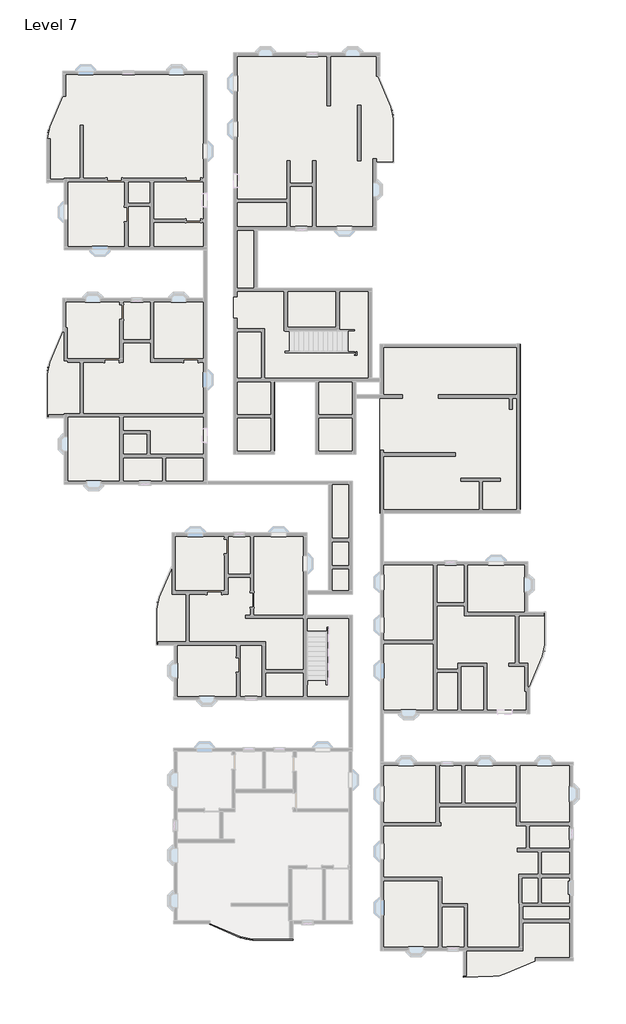
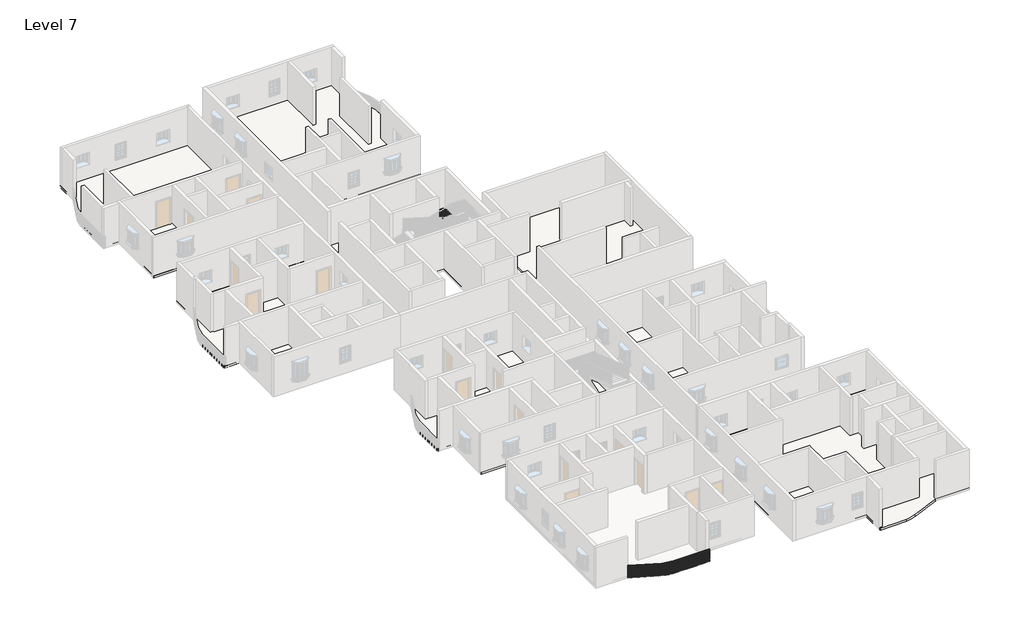
# One storey, part 5 of 14: 24 roofs, 1 railing.
"""IFC4 building model written with IfcOpenShell, lengths in millimetres."""

from ifc_helpers import new_model, si_unit, point, frame, frame_2d, origin, place, context, project, spatial, polyline, circle_curve, trimmed, segment, composite_curve, outline, extrude, element, save
from ifc_brep_helpers import plane_surface, cylinder_surface, revolved_surface, advanced_brep

model = new_model("IFC4")

# Units and contexts
model_context = context("Model", 3, world=origin())
ifc_project = project(units=[si_unit("LENGTHUNIT", "METRE", prefix="MILLI")], contexts=[model_context])

# Site, building, storey
site = spatial("IfcSite", under=ifc_project)
building = spatial("IfcBuilding", under=site)
storey = spatial("IfcBuildingStorey", under=building, Name="Level 7", Elevation=18288.0)

# Railing
placement = place(None, origin())
element("IfcRailing", 1, ObjectType="Handrail - Rectangular", at=placement, inside=storey, context=model_context, shape_type="SolidModel", body=[
    advanced_brep(
    [(-10014.8722294, -25076.9923935, 19202.4), (-10014.8722294, -25076.9923935, 19151.6), (-10034.8694485, -25123.6909077, 19151.6), (-10034.8694485, -25123.6909077, 19202.4), (-8065.5370278, -25911.7359335, 19202.4), (-8065.5370278, -25911.7359335, 19151.6), (-8085.5342469, -25958.4344477, 19151.6), (-8085.5342469, -25958.4344477, 19202.4), (-7315.6413127, -26065.5416506, 19151.6), (-7315.6413127, -26065.5416506, 19202.4), (-7315.6413127, -26116.3416506, 19151.6), (-7315.6413127, -26116.3416506, 19202.4), (-4746.0891351, -26065.5416506, 19202.4), (-4746.0891351, -26116.3416506, 19202.4), (-4746.0891351, -26116.3416506, 19151.6), (-4746.0891351, -26065.5416506, 19151.6)],
    [
        (0, 1),
        (1, 2),
        (2, 3),
        (3, 0),
        (0, 4),
        (4, 5),
        (5, 1),
        (5, 6),
        (6, 2),
        (6, 7),
        (7, 3),
        (7, 4),
        (8, 5, circle_curve(frame((-7315.6413127, -24160.5416506, 19151.6), z_axis=(0.0, 0.0, -1.0), x_axis=(-0.3936460446736572, -0.9192620907623599, 0.0)), 1905.0)),
        (4, 9, circle_curve(frame((-7315.6413127, -24160.5416506, 19202.4), z_axis=(0.0, 0.0, 1.0), x_axis=(-0.3936460446736572, -0.9192620907623599, 0.0)), 1905.0)),
        (9, 8),
        (10, 6, circle_curve(frame((-7315.6413127, -24160.5416506, 19151.6), z_axis=(0.0, 0.0, -1.0), x_axis=(-0.3936460446736572, -0.9192620907623599, 0.0)), 1955.8)),
        (8, 10),
        (11, 7, circle_curve(frame((-7315.6413127, -24160.5416506, 19202.4), z_axis=(0.0, 0.0, -1.0), x_axis=(-0.3936460446736572, -0.9192620907623599, 0.0)), 1955.8)),
        (10, 11),
        (11, 9),
        (12, 13),
        (13, 14),
        (14, 15),
        (15, 12),
        (9, 12),
        (15, 8),
        (14, 10),
        (13, 11),
    ],
    [
        plane_surface(frame((-10024.8708389, -25100.3416506, 19202.4), z_axis=(-0.9192620907623597, 0.39364604467365766, 0.0), x_axis=(0.39364604467365766, 0.9192620907623597, 0.0))),
        plane_surface(frame((-10014.8722294, -25076.9923935, 19202.4), z_axis=(0.3936460446736573, 0.9192620907623599, 0.0), x_axis=(0.9192620907623599, -0.3936460446736573, 0.0))),
        plane_surface(frame((-10014.8722294, -25076.9923935, 19151.6), z_axis=(0.0, 0.0, -1.0000000000000002), x_axis=(0.9192620907623599, -0.3936460446736573, 0.0))),
        plane_surface(frame((-10034.8694485, -25123.6909077, 19151.6), z_axis=(-0.39364604467365766, -0.9192620907623597, 0.0), x_axis=(0.9192620907623597, -0.39364604467365766, 0.0))),
        plane_surface(frame((-10034.8694485, -25123.6909077, 19202.4), z_axis=(0.0, 0.0, 1.0), x_axis=(0.9192620907623597, -0.39364604467365766, 0.0))),
        revolved_surface(polyline([(-8065.537027803317, -25911.735933502296, 19202.4), (-8065.537027803317, -25911.735933502296, 19151.6)]), (-7315.6413127, -24160.5416506, 19202.4), (0.0, 0.0, 1.0)),
        plane_surface(frame((-7315.6413127, -24160.5416506, 19151.6), z_axis=(0.0, 0.0, -1.0), x_axis=(-0.3936460446736572, -0.9192620907623599, 0.0))),
        cylinder_surface(frame((-7315.6413127, -24160.5416506, 19202.4), z_axis=(0.0, 0.0, 1.0), x_axis=(-0.3936460446736572, -0.9192620907623599, 0.0)), 1955.8),
        plane_surface(frame((-7315.6413127, -24160.5416506, 19202.4), z_axis=(0.0, 0.0, 1.0), x_axis=(-0.3936460446736572, -0.9192620907623599, 0.0))),
        plane_surface(frame((-4746.0891351, -26090.9416506, 19202.4), z_axis=(1.0, 0.0, 0.0), x_axis=(0.0, 1.0, 0.0))),
        plane_surface(frame((-7315.6413127, -26065.5416506, 19202.4), z_axis=(0.0, 1.0, 0.0), x_axis=(1.0, 0.0, 0.0))),
        plane_surface(frame((-7315.6413127, -26065.5416506, 19151.6), z_axis=(0.0, 0.0, -1.0), x_axis=(1.0, 0.0, 0.0))),
        plane_surface(frame((-7315.6413127, -26116.3416506, 19151.6), z_axis=(0.0, -1.0, 0.0), x_axis=(1.0, 0.0, 0.0))),
        plane_surface(frame((-7315.6413127, -26116.3416506, 19202.4), z_axis=(0.0, 0.0, 1.0), x_axis=(1.0, 0.0, 0.0))),
    ],
    [
        (0, [[1, 2, 3, 4]]),
        (1, [[-1, 5, 6, 7]]),
        (2, [[-2, -7, 8, 9]]),
        (3, [[-3, -9, 10, 11]]),
        (4, [[-4, -11, 12, -5]]),
        (5, [[13, -6, 14, 15]]),
        (6, [[16, -8, -13, 17]]),
        (7, [[18, -10, -16, 19]]),
        (8, [[-14, -12, -18, 20]]),
        (9, [[21, 22, 23, 24]]),
        (10, [[-15, 25, -24, 26]]),
        (11, [[-17, -26, -23, 27]]),
        (12, [[-19, -27, -22, 28]]),
        (13, [[-20, -28, -21, -25]]),
    ],
),
    extrude(outline(polyline([(-4785.1663127, -26100.4666506), (-4785.1663127, -26081.4166506), (-4766.1163127, -26081.4166506), (-4766.1163127, -26100.4666506), (-4785.1663127, -26100.4666506)])), frame((0.0, 0.0, 18288.0), z_axis=(0.0, 0.0, 1.0), x_axis=(1.0, 0.0, 0.0)), (0.0, 0.0, 1.0), 863.6),
    extrude(outline(polyline([(-4886.7663127, -26100.4666506), (-4886.7663127, -26081.4166506), (-4867.7163127, -26081.4166506), (-4867.7163127, -26100.4666506), (-4886.7663127, -26100.4666506)])), frame((0.0, 0.0, 18288.0), z_axis=(0.0, 0.0, 1.0), x_axis=(1.0, 0.0, 0.0)), (0.0, 0.0, 1.0), 863.6),
    extrude(outline(polyline([(-4988.3663127, -26100.4666506), (-4988.3663127, -26081.4166506), (-4969.3163127, -26081.4166506), (-4969.3163127, -26100.4666506), (-4988.3663127, -26100.4666506)])), frame((0.0, 0.0, 18288.0), z_axis=(0.0, 0.0, 1.0), x_axis=(1.0, 0.0, 0.0)), (0.0, 0.0, 1.0), 863.6),
    extrude(outline(polyline([(-5089.9663127, -26100.4666506), (-5089.9663127, -26081.4166506), (-5070.9163127, -26081.4166506), (-5070.9163127, -26100.4666506), (-5089.9663127, -26100.4666506)])), frame((0.0, 0.0, 18288.0), z_axis=(0.0, 0.0, 1.0), x_axis=(1.0, 0.0, 0.0)), (0.0, 0.0, 1.0), 863.6),
    extrude(outline(polyline([(-5191.5663127, -26100.4666506), (-5191.5663127, -26081.4166506), (-5172.5163127, -26081.4166506), (-5172.5163127, -26100.4666506), (-5191.5663127, -26100.4666506)])), frame((0.0, 0.0, 18288.0), z_axis=(0.0, 0.0, 1.0), x_axis=(1.0, 0.0, 0.0)), (0.0, 0.0, 1.0), 863.6),
    extrude(outline(polyline([(-5293.1663127, -26100.4666506), (-5293.1663127, -26081.4166506), (-5274.1163127, -26081.4166506), (-5274.1163127, -26100.4666506), (-5293.1663127, -26100.4666506)])), frame((0.0, 0.0, 18288.0), z_axis=(0.0, 0.0, 1.0), x_axis=(1.0, 0.0, 0.0)), (0.0, 0.0, 1.0), 863.6),
    extrude(outline(polyline([(-5394.7663127, -26100.4666506), (-5394.7663127, -26081.4166506), (-5375.7163127, -26081.4166506), (-5375.7163127, -26100.4666506), (-5394.7663127, -26100.4666506)])), frame((0.0, 0.0, 18288.0), z_axis=(0.0, 0.0, 1.0), x_axis=(1.0, 0.0, 0.0)), (0.0, 0.0, 1.0), 863.6),
    extrude(outline(polyline([(-5496.3663127, -26100.4666506), (-5496.3663127, -26081.4166506), (-5477.3163127, -26081.4166506), (-5477.3163127, -26100.4666506), (-5496.3663127, -26100.4666506)])), frame((0.0, 0.0, 18288.0), z_axis=(0.0, 0.0, 1.0), x_axis=(1.0, 0.0, 0.0)), (0.0, 0.0, 1.0), 863.6),
    extrude(outline(polyline([(-5597.9663127, -26100.4666506), (-5597.9663127, -26081.4166506), (-5578.9163127, -26081.4166506), (-5578.9163127, -26100.4666506), (-5597.9663127, -26100.4666506)])), frame((0.0, 0.0, 18288.0), z_axis=(0.0, 0.0, 1.0), x_axis=(1.0, 0.0, 0.0)), (0.0, 0.0, 1.0), 863.6),
    extrude(outline(polyline([(-5699.5663127, -26100.4666506), (-5699.5663127, -26081.4166506), (-5680.5163127, -26081.4166506), (-5680.5163127, -26100.4666506), (-5699.5663127, -26100.4666506)])), frame((0.0, 0.0, 18288.0), z_axis=(0.0, 0.0, 1.0), x_axis=(1.0, 0.0, 0.0)), (0.0, 0.0, 1.0), 863.6),
    extrude(outline(polyline([(-5801.1663127, -26100.4666506), (-5801.1663127, -26081.4166506), (-5782.1163127, -26081.4166506), (-5782.1163127, -26100.4666506), (-5801.1663127, -26100.4666506)])), frame((0.0, 0.0, 18288.0), z_axis=(0.0, 0.0, 1.0), x_axis=(1.0, 0.0, 0.0)), (0.0, 0.0, 1.0), 863.6),
    extrude(outline(polyline([(-5902.7663127, -26100.4666506), (-5902.7663127, -26081.4166506), (-5883.7163127, -26081.4166506), (-5883.7163127, -26100.4666506), (-5902.7663127, -26100.4666506)])), frame((0.0, 0.0, 18288.0), z_axis=(0.0, 0.0, 1.0), x_axis=(1.0, 0.0, 0.0)), (0.0, 0.0, 1.0), 863.6),
    extrude(outline(polyline([(-6004.3663127, -26100.4666506), (-6004.3663127, -26081.4166506), (-5985.3163127, -26081.4166506), (-5985.3163127, -26100.4666506), (-6004.3663127, -26100.4666506)])), frame((0.0, 0.0, 18288.0), z_axis=(0.0, 0.0, 1.0), x_axis=(1.0, 0.0, 0.0)), (0.0, 0.0, 1.0), 863.6),
    extrude(outline(polyline([(-6105.9663127, -26100.4666506), (-6105.9663127, -26081.4166506), (-6086.9163127, -26081.4166506), (-6086.9163127, -26100.4666506), (-6105.9663127, -26100.4666506)])), frame((0.0, 0.0, 18288.0), z_axis=(0.0, 0.0, 1.0), x_axis=(1.0, 0.0, 0.0)), (0.0, 0.0, 1.0), 863.6),
    extrude(outline(polyline([(-6207.5663127, -26100.4666506), (-6207.5663127, -26081.4166506), (-6188.5163127, -26081.4166506), (-6188.5163127, -26100.4666506), (-6207.5663127, -26100.4666506)])), frame((0.0, 0.0, 18288.0), z_axis=(0.0, 0.0, 1.0), x_axis=(1.0, 0.0, 0.0)), (0.0, 0.0, 1.0), 863.6),
    extrude(outline(polyline([(-6309.1663127, -26100.4666506), (-6309.1663127, -26081.4166506), (-6290.1163127, -26081.4166506), (-6290.1163127, -26100.4666506), (-6309.1663127, -26100.4666506)])), frame((0.0, 0.0, 18288.0), z_axis=(0.0, 0.0, 1.0), x_axis=(1.0, 0.0, 0.0)), (0.0, 0.0, 1.0), 863.6),
    extrude(outline(polyline([(-6410.7663127, -26100.4666506), (-6410.7663127, -26081.4166506), (-6391.7163127, -26081.4166506), (-6391.7163127, -26100.4666506), (-6410.7663127, -26100.4666506)])), frame((0.0, 0.0, 18288.0), z_axis=(0.0, 0.0, 1.0), x_axis=(1.0, 0.0, 0.0)), (0.0, 0.0, 1.0), 863.6),
    extrude(outline(polyline([(-6512.3663127, -26100.4666506), (-6512.3663127, -26081.4166506), (-6493.3163127, -26081.4166506), (-6493.3163127, -26100.4666506), (-6512.3663127, -26100.4666506)])), frame((0.0, 0.0, 18288.0), z_axis=(0.0, 0.0, 1.0), x_axis=(1.0, 0.0, 0.0)), (0.0, 0.0, 1.0), 863.6),
    extrude(outline(polyline([(-6613.9663127, -26100.4666506), (-6613.9663127, -26081.4166506), (-6594.9163127, -26081.4166506), (-6594.9163127, -26100.4666506), (-6613.9663127, -26100.4666506)])), frame((0.0, 0.0, 18288.0), z_axis=(0.0, 0.0, 1.0), x_axis=(1.0, 0.0, 0.0)), (0.0, 0.0, 1.0), 863.6),
    extrude(outline(polyline([(-6715.5663127, -26100.4666506), (-6715.5663127, -26081.4166506), (-6696.5163127, -26081.4166506), (-6696.5163127, -26100.4666506), (-6715.5663127, -26100.4666506)])), frame((0.0, 0.0, 18288.0), z_axis=(0.0, 0.0, 1.0), x_axis=(1.0, 0.0, 0.0)), (0.0, 0.0, 1.0), 863.6),
    extrude(outline(polyline([(-6817.1663127, -26100.4666506), (-6817.1663127, -26081.4166506), (-6798.1163127, -26081.4166506), (-6798.1163127, -26100.4666506), (-6817.1663127, -26100.4666506)])), frame((0.0, 0.0, 18288.0), z_axis=(0.0, 0.0, 1.0), x_axis=(1.0, 0.0, 0.0)), (0.0, 0.0, 1.0), 863.6),
    extrude(outline(polyline([(-6918.7663127, -26100.4666506), (-6918.7663127, -26081.4166506), (-6899.7163127, -26081.4166506), (-6899.7163127, -26100.4666506), (-6918.7663127, -26100.4666506)])), frame((0.0, 0.0, 18288.0), z_axis=(0.0, 0.0, 1.0), x_axis=(1.0, 0.0, 0.0)), (0.0, 0.0, 1.0), 863.6),
    extrude(outline(polyline([(-7020.3663127, -26100.4666506), (-7020.3663127, -26081.4166506), (-7001.3163127, -26081.4166506), (-7001.3163127, -26100.4666506), (-7020.3663127, -26100.4666506)])), frame((0.0, 0.0, 18288.0), z_axis=(0.0, 0.0, 1.0), x_axis=(1.0, 0.0, 0.0)), (0.0, 0.0, 1.0), 863.6),
    extrude(outline(polyline([(-7121.9663127, -26100.4666506), (-7121.9663127, -26081.4166506), (-7102.9163127, -26081.4166506), (-7102.9163127, -26100.4666506), (-7121.9663127, -26100.4666506)])), frame((0.0, 0.0, 18288.0), z_axis=(0.0, 0.0, 1.0), x_axis=(1.0, 0.0, 0.0)), (0.0, 0.0, 1.0), 863.6),
    extrude(outline(polyline([(-7223.5663127, -26100.4666506), (-7223.5663127, -26081.4166506), (-7204.5163127, -26081.4166506), (-7204.5163127, -26100.4666506), (-7223.5663127, -26100.4666506)])), frame((0.0, 0.0, 18288.0), z_axis=(0.0, 0.0, 1.0), x_axis=(1.0, 0.0, 0.0)), (0.0, 0.0, 1.0), 863.6),
    extrude(outline(polyline([(-7395.3185803, -26098.8530973), (-7394.6296262, -26079.8155596), (-7375.5920885, -26080.5045137), (-7376.2810426, -26099.5420514), (-7395.3185803, -26098.8530973)])), frame((0.0, 0.0, 18288.0), z_axis=(0.0, 0.0, 1.0), x_axis=(1.0, 0.0, 0.0)), (0.0, 0.0, 1.0), 863.6),
    extrude(outline(polyline([(-7497.177549, -26091.9774704), (-7495.4880357, -26073.0025384), (-7476.5131037, -26074.6920517), (-7478.2026169, -26093.6669837), (-7497.177549, -26091.9774704)])), frame((0.0, 0.0, 18288.0), z_axis=(0.0, 0.0, 1.0), x_axis=(1.0, 0.0, 0.0)), (0.0, 0.0, 1.0), 863.6),
    extrude(outline(polyline([(-7598.5337632, -26079.7528408), (-7595.8483698, -26060.8930645), (-7576.9885935, -26063.5784579), (-7579.6739869, -26082.4382342), (-7598.5337632, -26079.7528408)])), frame((0.0, 0.0, 18288.0), z_axis=(0.0, 0.0, 1.0), x_axis=(1.0, 0.0, 0.0)), (0.0, 0.0, 1.0), 863.6),
    extrude(outline(polyline([(-7699.1065227, -26062.2130639), (-7695.4326862, -26043.5206744), (-7676.7402967, -26047.1945108), (-7680.4141332, -26065.8869003), (-7699.1065227, -26062.2130639)])), frame((0.0, 0.0, 18288.0), z_axis=(0.0, 0.0, 1.0), x_axis=(1.0, 0.0, 0.0)), (0.0, 0.0, 1.0), 863.6),
    extrude(outline(polyline([(-7798.6172969, -26039.4067149), (-7793.9651918, -26020.9334797), (-7775.4919566, -26025.5855848), (-7780.1440617, -26044.05882), (-7798.6172969, -26039.4067149)])), frame((0.0, 0.0, 18288.0), z_axis=(0.0, 0.0, 1.0), x_axis=(1.0, 0.0, 0.0)), (0.0, 0.0, 1.0), 863.6),
    extrude(outline(polyline([(-7896.7904963, -26011.396955), (-7891.1730064, -25993.1940347), (-7872.9700861, -25998.8115246), (-7878.587576, -26017.0144449), (-7896.7904963, -26011.396955)])), frame((0.0, 0.0, 18288.0), z_axis=(0.0, 0.0, 1.0), x_axis=(1.0, 0.0, 0.0)), (0.0, 0.0, 1.0), 863.6),
    extrude(outline(polyline([(-7993.3542357, -25978.2613554), (-7986.7869183, -25960.379162), (-7968.9047249, -25966.9464794), (-7975.4720423, -25984.8286729), (-7993.3542357, -25978.2613554)])), frame((0.0, 0.0, 18288.0), z_axis=(0.0, 0.0, 1.0), x_axis=(1.0, 0.0, 0.0)), (0.0, 0.0, 1.0), 863.6),
    extrude(outline(polyline([(-8169.4357205, -25905.2369062), (-8161.9367633, -25887.7249634), (-8144.4248205, -25895.2239205), (-8151.9237777, -25912.7358634), (-8169.4357205, -25905.2369062)])), frame((0.0, 0.0, 18288.0), z_axis=(0.0, 0.0, 1.0), x_axis=(1.0, 0.0, 0.0)), (0.0, 0.0, 1.0), 863.6),
    extrude(outline(polyline([(-8262.8327489, -25865.2424681), (-8255.3337918, -25847.7305252), (-8237.8218489, -25855.2294824), (-8245.3208061, -25872.7414252), (-8262.8327489, -25865.2424681)])), frame((0.0, 0.0, 18288.0), z_axis=(0.0, 0.0, 1.0), x_axis=(1.0, 0.0, 0.0)), (0.0, 0.0, 1.0), 863.6),
    extrude(outline(polyline([(-8356.2297773, -25825.2480299), (-8348.7308202, -25807.7360871), (-8331.2188774, -25815.2350443), (-8338.7178345, -25832.7469871), (-8356.2297773, -25825.2480299)])), frame((0.0, 0.0, 18288.0), z_axis=(0.0, 0.0, 1.0), x_axis=(1.0, 0.0, 0.0)), (0.0, 0.0, 1.0), 863.6),
    extrude(outline(polyline([(-8449.6268058, -25785.2535918), (-8442.1278486, -25767.741649), (-8424.6159058, -25775.2406061), (-8432.1148629, -25792.752549), (-8449.6268058, -25785.2535918)])), frame((0.0, 0.0, 18288.0), z_axis=(0.0, 0.0, 1.0), x_axis=(1.0, 0.0, 0.0)), (0.0, 0.0, 1.0), 863.6),
    extrude(outline(polyline([(-8543.0238342, -25745.2591537), (-8535.524877, -25727.7472108), (-8518.0129342, -25735.246168), (-8525.5118914, -25752.7581108), (-8543.0238342, -25745.2591537)])), frame((0.0, 0.0, 18288.0), z_axis=(0.0, 0.0, 1.0), x_axis=(1.0, 0.0, 0.0)), (0.0, 0.0, 1.0), 863.6),
    extrude(outline(polyline([(-8636.4208626, -25705.2647155), (-8628.9219055, -25687.7527727), (-8611.4099626, -25695.2517298), (-8618.9089198, -25712.7636727), (-8636.4208626, -25705.2647155)])), frame((0.0, 0.0, 18288.0), z_axis=(0.0, 0.0, 1.0), x_axis=(1.0, 0.0, 0.0)), (0.0, 0.0, 1.0), 863.6),
    extrude(outline(polyline([(-8729.817891, -25665.2702774), (-8722.3189339, -25647.7583346), (-8704.806991, -25655.2572917), (-8712.3059482, -25672.7692345), (-8729.817891, -25665.2702774)])), frame((0.0, 0.0, 18288.0), z_axis=(0.0, 0.0, 1.0), x_axis=(1.0, 0.0, 0.0)), (0.0, 0.0, 1.0), 863.6),
    extrude(outline(polyline([(-8823.2149194, -25625.2758392), (-8815.7159623, -25607.7638964), (-8798.2040195, -25615.2628536), (-8805.7029766, -25632.7747964), (-8823.2149194, -25625.2758392)])), frame((0.0, 0.0, 18288.0), z_axis=(0.0, 0.0, 1.0), x_axis=(1.0, 0.0, 0.0)), (0.0, 0.0, 1.0), 863.6),
    extrude(outline(polyline([(-8916.6119479, -25585.2814011), (-8909.1129907, -25567.7694583), (-8891.6010479, -25575.2684154), (-8899.100005, -25592.7803583), (-8916.6119479, -25585.2814011)])), frame((0.0, 0.0, 18288.0), z_axis=(0.0, 0.0, 1.0), x_axis=(1.0, 0.0, 0.0)), (0.0, 0.0, 1.0), 863.6),
    extrude(outline(polyline([(-9010.0089763, -25545.286963), (-9002.5100191, -25527.7750201), (-8984.9980763, -25535.2739773), (-8992.4970335, -25552.7859201), (-9010.0089763, -25545.286963)])), frame((0.0, 0.0, 18288.0), z_axis=(0.0, 0.0, 1.0), x_axis=(1.0, 0.0, 0.0)), (0.0, 0.0, 1.0), 863.6),
    extrude(outline(polyline([(-9103.4060047, -25505.2925248), (-9095.9070476, -25487.780582), (-9078.3951047, -25495.2795391), (-9085.8940619, -25512.791482), (-9103.4060047, -25505.2925248)])), frame((0.0, 0.0, 18288.0), z_axis=(0.0, 0.0, 1.0), x_axis=(1.0, 0.0, 0.0)), (0.0, 0.0, 1.0), 863.6),
    extrude(outline(polyline([(-9196.8030331, -25465.2980867), (-9189.304076, -25447.7861439), (-9171.7921332, -25455.285101), (-9179.2910903, -25472.7970438), (-9196.8030331, -25465.2980867)])), frame((0.0, 0.0, 18288.0), z_axis=(0.0, 0.0, 1.0), x_axis=(1.0, 0.0, 0.0)), (0.0, 0.0, 1.0), 863.6),
    extrude(outline(polyline([(-9290.2000616, -25425.3036485), (-9282.7011044, -25407.7917057), (-9265.1891616, -25415.2906629), (-9272.6881187, -25432.8026057), (-9290.2000616, -25425.3036485)])), frame((0.0, 0.0, 18288.0), z_axis=(0.0, 0.0, 1.0), x_axis=(1.0, 0.0, 0.0)), (0.0, 0.0, 1.0), 863.6),
    extrude(outline(polyline([(-9383.59709, -25385.3092104), (-9376.0981328, -25367.7972676), (-9358.58619, -25375.2962247), (-9366.0851471, -25392.8081676), (-9383.59709, -25385.3092104)])), frame((0.0, 0.0, 18288.0), z_axis=(0.0, 0.0, 1.0), x_axis=(1.0, 0.0, 0.0)), (0.0, 0.0, 1.0), 863.6),
    extrude(outline(polyline([(-9476.9941184, -25345.3147723), (-9469.4951612, -25327.8028294), (-9451.9832184, -25335.3017866), (-9459.4821756, -25352.8137294), (-9476.9941184, -25345.3147723)])), frame((0.0, 0.0, 18288.0), z_axis=(0.0, 0.0, 1.0), x_axis=(1.0, 0.0, 0.0)), (0.0, 0.0, 1.0), 863.6),
    extrude(outline(polyline([(-9570.3911468, -25305.3203341), (-9562.8921897, -25287.8083913), (-9545.3802468, -25295.3073485), (-9552.879204, -25312.8192913), (-9570.3911468, -25305.3203341)])), frame((0.0, 0.0, 18288.0), z_axis=(0.0, 0.0, 1.0), x_axis=(1.0, 0.0, 0.0)), (0.0, 0.0, 1.0), 863.6),
    extrude(outline(polyline([(-9663.7881752, -25265.325896), (-9656.2892181, -25247.8139532), (-9638.7772753, -25255.3129103), (-9646.2762324, -25272.8248531), (-9663.7881752, -25265.325896)])), frame((0.0, 0.0, 18288.0), z_axis=(0.0, 0.0, 1.0), x_axis=(1.0, 0.0, 0.0)), (0.0, 0.0, 1.0), 863.6),
    extrude(outline(polyline([(-9757.1852037, -25225.3314579), (-9749.6862465, -25207.819515), (-9732.1743037, -25215.3184722), (-9739.6732608, -25232.830415), (-9757.1852037, -25225.3314579)])), frame((0.0, 0.0, 18288.0), z_axis=(0.0, 0.0, 1.0), x_axis=(1.0, 0.0, 0.0)), (0.0, 0.0, 1.0), 863.6),
    extrude(outline(polyline([(-9850.5822321, -25185.3370197), (-9843.0832749, -25167.8250769), (-9825.5713321, -25175.324034), (-9833.0702893, -25192.8359769), (-9850.5822321, -25185.3370197)])), frame((0.0, 0.0, 18288.0), z_axis=(0.0, 0.0, 1.0), x_axis=(1.0, 0.0, 0.0)), (0.0, 0.0, 1.0), 863.6),
    extrude(outline(polyline([(-9943.9792605, -25145.3425816), (-9936.4803034, -25127.8306387), (-9918.9683605, -25135.3295959), (-9926.4673177, -25152.8415387), (-9943.9792605, -25145.3425816)])), frame((0.0, 0.0, 18288.0), z_axis=(0.0, 0.0, 1.0), x_axis=(1.0, 0.0, 0.0)), (0.0, 0.0, 1.0), 863.6),
    extrude(outline(polyline([(-7325.1663127, -26100.4666506), (-7325.1663127, -26081.4166506), (-7306.1163127, -26081.4166506), (-7306.1163127, -26100.4666506), (-7325.1663127, -26100.4666506)])), frame((0.0, 0.0, 18288.0), z_axis=(0.0, 0.0, 1.0), x_axis=(1.0, 0.0, 0.0)), (0.0, 0.0, 1.0), 863.6),
    extrude(outline(polyline([(-8088.0410874, -25940.0916834), (-8080.5421302, -25922.5797406), (-8063.0301874, -25930.0786978), (-8070.5291445, -25947.5906406), (-8088.0410874, -25940.0916834)])), frame((0.0, 0.0, 18288.0), z_axis=(0.0, 0.0, 1.0), x_axis=(1.0, 0.0, 0.0)), (0.0, 0.0, 1.0), 863.6),
    extrude(outline(polyline([(-4765.1391351, -26100.4666506), (-4765.1391351, -26081.4166506), (-4746.0891351, -26081.4166506), (-4746.0891351, -26100.4666506), (-4765.1391351, -26100.4666506)])), frame((0.0, 0.0, 18288.0), z_axis=(0.0, 0.0, 1.0), x_axis=(1.0, 0.0, 0.0)), (0.0, 0.0, 1.0), 863.6),
    extrude(outline(polyline([(-10028.6203175, -25109.097622), (-10021.1213604, -25091.5856792), (-10003.6094175, -25099.0846363), (-10011.1083747, -25116.5965792), (-10028.6203175, -25109.097622)])), frame((0.0, 0.0, 18288.0), z_axis=(0.0, 0.0, 1.0), x_axis=(1.0, 0.0, 0.0)), (0.0, 0.0, 1.0), 863.6),
])

# Roofs
element("IfcRoof", 2, ObjectType="Generic - 12\"", at=placement, inside=storey, context=model_context, shape_type="SweptSolid", body=[
    extrude(outline(composite_curve([segment(polyline([(6070.4380523, -26783.9042694), (812.6380523, -26783.9042694), (812.6380523, -14845.9042694), (13017.3380523, -14845.9042694), (13017.3380523, -27431.6042694), (10660.5280667, -27431.6042694), (8711.1928652, -28266.3478094)]), True, "CONTINUOUS"), segment(trimmed(circle_curve(frame_2d((7951.2985405, -26491.8042694)), 1930.4), [point((8711.1928652, -28266.3478094))], [point((7953.0959373, -28422.2034326))], False, "CARTESIAN"), True, "CONTINUOUS"), segment(polyline([(7953.0959373, -28422.2034326), (6070.4380523, -28487.9472947), (6070.4380523, -26783.9042694)]), True, "CONTINUOUS")], self_intersect=False)), frame((0.0, 0.0, 18288.0), z_axis=(0.0, 0.0, 1.0), x_axis=(1.0, 0.0, 0.0)), (0.0, 0.0, 1.0), 152.4),
])
element("IfcRoof", 3, ObjectType="Generic - 12\"", at=placement, inside=storey, context=model_context, shape_type="SweptSolid", body=[
    extrude(outline(composite_curve([segment(polyline([(10274.1380523, -11759.8042694), (803.8108649, -11759.8042694), (803.8108649, -2133.2042694), (10159.8380523, -2133.2042694), (10159.8380523, -5352.6542694), (11264.7380523, -5352.6542694), (11264.7380523, -7397.5810633)]), True, "CONTINUOUS"), segment(trimmed(circle_curve(frame_2d((9334.3380523, -7397.5810633)), 1930.4), [point((11264.7380523, -7397.5810633))], [point((11108.8815923, -8157.475388))], False, "CARTESIAN"), True, "CONTINUOUS"), segment(polyline([(11108.8815923, -8157.475388), (10274.1380523, -10106.8105895), (10274.1380523, -11759.8042694)]), True, "CONTINUOUS")], self_intersect=False)), frame((0.0, 0.0, 18288.0), z_axis=(0.0, 0.0, 1.0), x_axis=(1.0, 0.0, 0.0)), (0.0, 0.0, 1.0), 152.4),
])
element("IfcRoof", 4, ObjectType="Generic - 12\"", at=placement, inside=storey, context=model_context, shape_type="SweptSolid", body=[
    extrude(outline(composite_curve([segment(polyline([(-13395.387215, -7421.9416506), (-13395.387215, -5140.4900045)]), True, "CONTINUOUS"), segment(trimmed(circle_curve(frame_2d((-11464.987215, -5140.4900045)), 1930.4), [point((-13395.387215, -5140.4900045))], [point((-13239.530755, -4380.5956799))], False, "CARTESIAN"), True, "CONTINUOUS"), segment(polyline([(-13239.530755, -4380.5956799), (-12404.787215, -2431.2604783), (-12404.787215, -322.6416506), (-3857.687215, -322.6416506), (-3857.687215, -5523.2916506), (-974.1891351, -5523.2916506), (-974.1891351, -10889.0416506), (-12290.487215, -10889.0416506), (-12290.487215, -7421.9416506), (-13395.387215, -7421.9416506)]), True, "CONTINUOUS")], self_intersect=False)), frame((0.0, 0.0, 18288.0), z_axis=(0.0, 0.0, 1.0), x_axis=(1.0, 0.0, 0.0)), (0.0, 0.0, 1.0), 152.4),
])
element("IfcRoof", 5, ObjectType="Generic - 12\"", at=placement, inside=storey, context=model_context, shape_type="SweptSolid", body=[
    extrude(outline(polyline([(-2472.7891351, 2953.9583494), (-961.4891351, 2953.9583494), (-961.4891351, -4202.4916506), (-2472.7891351, -4202.4916506), (-2472.7891351, 2953.9583494)])), frame((0.0, 0.0, 18288.0), z_axis=(0.0, 0.0, 1.0), x_axis=(1.0, 0.0, 0.0)), (0.0, 0.0, 1.0), 152.4),
])
element("IfcRoof", 6, ObjectType="Generic - 12\"", at=placement, inside=storey, context=model_context, shape_type="SweptSolid", body=[
    extrude(outline(composite_curve([segment(polyline([(-10194.3891351, 2750.7583494), (-19236.7891351, 2750.7583494), (-19236.7891351, 6979.8583494), (-20341.6891351, 6979.8583494), (-20341.6891351, 9746.7948172)]), True, "CONTINUOUS"), segment(trimmed(circle_curve(frame_2d((-18411.2891351, 9746.7948172)), 1930.4), [point((-20341.6891351, 9746.7948172))], [point((-20185.8326751, 10506.6891419))], False, "CARTESIAN"), True, "CONTINUOUS"), segment(polyline([(-20185.8326751, 10506.6891419), (-19351.0891351, 12456.0243434), (-19351.0891351, 14536.3583494), (-10194.3891351, 14536.3583494), (-10194.3891351, 2750.7583494)]), True, "CONTINUOUS")], self_intersect=False)), frame((0.0, 0.0, 18288.0), z_axis=(0.0, 0.0, 1.0), x_axis=(1.0, 0.0, 0.0)), (0.0, 0.0, 1.0), 152.4),
])
element("IfcRoof", 7, ObjectType="Generic - 12\"", at=placement, inside=storey, context=model_context, shape_type="SweptSolid", body=[
    extrude(outline(composite_curve([segment(polyline([(-10194.3891351, 17609.7583494), (-19236.7891351, 17609.7583494), (-19236.7891351, 21889.6583494), (-20341.6891351, 21889.6583494), (-20341.6891351, 24656.5948172)]), True, "CONTINUOUS"), segment(trimmed(circle_curve(frame_2d((-18411.2891351, 24656.5948172)), 1930.4), [point((-20341.6891351, 24656.5948172))], [point((-20185.8326751, 25416.4891419))], False, "CARTESIAN"), True, "CONTINUOUS"), segment(polyline([(-20185.8326751, 25416.4891419), (-19351.0891351, 27365.8243434), (-19351.0891351, 28950.8583494), (-10194.3891351, 28950.8583494), (-10194.3891351, 17609.7583494)]), True, "CONTINUOUS")], self_intersect=False)), frame((0.0, 0.0, 18288.0), z_axis=(0.0, 0.0, 1.0), x_axis=(1.0, 0.0, 0.0)), (0.0, 0.0, 1.0), 152.4),
])
element("IfcRoof", 8, ObjectType="Generic - 12\"", at=placement, inside=storey, context=model_context, shape_type="SweptSolid", body=[
    extrude(outline(composite_curve([segment(polyline([(-8492.5891351, 18875.1215905), (-8492.5891351, 30101.9215905), (664.1108649, 30101.9215905), (664.1108649, 28631.1875845), (1498.8544049, 26681.8523829)]), True, "CONTINUOUS"), segment(trimmed(circle_curve(frame_2d((-275.6891351, 25921.9580583)), 1930.4), [point((1498.8544049, 26681.8523829))], [point((1654.7108649, 25921.9580583))], False, "CARTESIAN"), True, "CONTINUOUS"), segment(polyline([(1654.7108649, 25921.9580583), (1654.7108649, 23155.0215905), (549.8108649, 23155.0215905), (549.8108649, 18875.1215905), (-8492.5891351, 18875.1215905)]), True, "CONTINUOUS")], self_intersect=False)), frame((0.0, 0.0, 18288.0), z_axis=(0.0, 0.0, 1.0), x_axis=(1.0, 0.0, 0.0)), (0.0, 0.0, 1.0), 152.4),
])
element("IfcRoof", 9, ObjectType="Generic - 12\"", at=placement, inside=storey, context=model_context, shape_type="SweptSolid", body=[
    extrude(outline(polyline([(-8492.5891351, 9478.4949943), (-5914.4891351, 9478.4949943), (-5914.4891351, 4665.1949943), (-8492.5891351, 4665.1949943), (-8492.5891351, 9478.4949943)])), frame((0.0, 0.0, 18288.0), z_axis=(0.0, 0.0, 1.0), x_axis=(1.0, 0.0, 0.0)), (0.0, 0.0, 1.0), 152.4),
])
element("IfcRoof", 10, ObjectType="Generic - 12\"", at=placement, inside=storey, context=model_context, shape_type="SweptSolid", body=[
    extrude(outline(polyline([(-3310.9891351, 9478.4949943), (-745.5891351, 9478.4949943), (-745.5891351, 4652.4949943), (-3310.9891351, 4652.4949943), (-3310.9891351, 9478.4949943)])), frame((0.0, 0.0, 18288.0), z_axis=(0.0, 0.0, 1.0), x_axis=(1.0, 0.0, 0.0)), (0.0, 0.0, 1.0), 152.4),
])
element("IfcRoof", 11, ObjectType="Generic - 12\"", at=placement, inside=storey, context=model_context, shape_type="SweptSolid", body=[
    extrude(outline(polyline([(-8492.5891351, 19078.3215905), (-6993.9891351, 19078.3215905), (-6993.9891351, 14988.9215905), (-8492.5891351, 14988.9215905), (-8492.5891351, 19078.3215905)])), frame((0.0, 0.0, 18288.0), z_axis=(0.0, 0.0, 1.0), x_axis=(1.0, 0.0, 0.0)), (0.0, 0.0, 1.0), 152.4),
])
element("IfcRoof", 12, ObjectType="Generic - 12\"", at=placement, inside=storey, context=model_context, shape_type="SweptSolid", body=[
    extrude(outline(polyline([(-8492.5891351, 15192.1215905), (257.7108649, 15192.1215905), (257.7108649, 9275.2949943), (-8492.5891351, 9275.2949943), (-8492.5891351, 15192.1215905)])), frame((0.0, 0.0, 18288.0), z_axis=(0.0, 0.0, 1.0), x_axis=(1.0, 0.0, 0.0)), (0.0, 0.0, 1.0), 152.4),
])
element("IfcRoof", 13, ObjectType="Generic - 12\"", at=placement, inside=storey, context=model_context, shape_type="SweptSolid", body=[
    extrude(outline(polyline([(793.5880523, 11646.2957306), (9677.2380523, 11646.2957306), (9677.2380523, 940.1957306), (793.5880523, 940.1957306), (793.5880523, 11646.2957306)])), frame((0.0, 0.0, 18288.0), z_axis=(0.0, 0.0, 1.0), x_axis=(1.0, 0.0, 0.0)), (0.0, 0.0, 1.0), 152.4),
])
element("IfcRoof", 14, ObjectType="Generic - 12\"", at=placement, inside=storey, context=model_context, shape_type="SweptSolid", body=[
    extrude(outline(composite_curve([segment(polyline([(6070.4380523, -26783.9042694), (812.6380523, -26783.9042694), (812.6380523, -14845.9042694), (13017.3380523, -14845.9042694), (13017.3380523, -27431.6042694), (10660.5280667, -27431.6042694), (8711.1928652, -28266.3478094)]), True, "CONTINUOUS"), segment(trimmed(circle_curve(frame_2d((7951.2985405, -26491.8042694)), 1930.4), [point((8711.1928652, -28266.3478094))], [point((7953.0959373, -28422.2034326))], False, "CARTESIAN"), True, "CONTINUOUS"), segment(polyline([(7953.0959373, -28422.2034326), (6070.4380523, -28487.9472947), (6070.4380523, -26783.9042694)]), True, "CONTINUOUS")], self_intersect=False)), frame((0.0, 0.0, 18288.0), z_axis=(0.0, 0.0, 1.0), x_axis=(1.0, 0.0, 0.0)), (0.0, 0.0, 1.0), 152.4),
])
element("IfcRoof", 15, ObjectType="Generic - 12\"", at=placement, inside=storey, context=model_context, shape_type="SweptSolid", body=[
    extrude(outline(composite_curve([segment(polyline([(10274.1380523, -11759.8042694), (803.8108649, -11759.8042694), (803.8108649, -2133.2042694), (10159.8380523, -2133.2042694), (10159.8380523, -5352.6542694), (11264.7380523, -5352.6542694), (11264.7380523, -7397.5810633)]), True, "CONTINUOUS"), segment(trimmed(circle_curve(frame_2d((9334.3380523, -7397.5810633)), 1930.4), [point((11264.7380523, -7397.5810633))], [point((11108.8815923, -8157.475388))], False, "CARTESIAN"), True, "CONTINUOUS"), segment(polyline([(11108.8815923, -8157.475388), (10274.1380523, -10106.8105895), (10274.1380523, -11759.8042694)]), True, "CONTINUOUS")], self_intersect=False)), frame((0.0, 0.0, 18288.0), z_axis=(0.0, 0.0, 1.0), x_axis=(1.0, 0.0, 0.0)), (0.0, 0.0, 1.0), 152.4),
])
element("IfcRoof", 16, ObjectType="Generic - 12\"", at=placement, inside=storey, context=model_context, shape_type="SweptSolid", body=[
    extrude(outline(composite_curve([segment(polyline([(-13395.387215, -7421.9416506), (-13395.387215, -5140.4900045)]), True, "CONTINUOUS"), segment(trimmed(circle_curve(frame_2d((-11464.987215, -5140.4900045)), 1930.4), [point((-13395.387215, -5140.4900045))], [point((-13239.530755, -4380.5956799))], False, "CARTESIAN"), True, "CONTINUOUS"), segment(polyline([(-13239.530755, -4380.5956799), (-12404.787215, -2431.2604783), (-12404.787215, -322.6416506), (-3857.687215, -322.6416506), (-3857.687215, -5523.2916506), (-974.1891351, -5523.2916506), (-974.1891351, -10889.0416506), (-12290.487215, -10889.0416506), (-12290.487215, -7421.9416506), (-13395.387215, -7421.9416506)]), True, "CONTINUOUS")], self_intersect=False)), frame((0.0, 0.0, 18288.0), z_axis=(0.0, 0.0, 1.0), x_axis=(1.0, 0.0, 0.0)), (0.0, 0.0, 1.0), 152.4),
])
element("IfcRoof", 17, ObjectType="Generic - 12\"", at=placement, inside=storey, context=model_context, shape_type="SweptSolid", body=[
    extrude(outline(polyline([(-2472.7891351, 2953.9583494), (-961.4891351, 2953.9583494), (-961.4891351, -4202.4916506), (-2472.7891351, -4202.4916506), (-2472.7891351, 2953.9583494)])), frame((0.0, 0.0, 18288.0), z_axis=(0.0, 0.0, 1.0), x_axis=(1.0, 0.0, 0.0)), (0.0, 0.0, 1.0), 152.4),
])
element("IfcRoof", 18, ObjectType="Generic - 12\"", at=placement, inside=storey, context=model_context, shape_type="SweptSolid", body=[
    extrude(outline(composite_curve([segment(polyline([(-10194.3891351, 2750.7583494), (-19236.7891351, 2750.7583494), (-19236.7891351, 6979.8583494), (-20341.6891351, 6979.8583494), (-20341.6891351, 9746.7948172)]), True, "CONTINUOUS"), segment(trimmed(circle_curve(frame_2d((-18411.2891351, 9746.7948172)), 1930.4), [point((-20341.6891351, 9746.7948172))], [point((-20185.8326751, 10506.6891419))], False, "CARTESIAN"), True, "CONTINUOUS"), segment(polyline([(-20185.8326751, 10506.6891419), (-19351.0891351, 12456.0243434), (-19351.0891351, 14536.3583494), (-10194.3891351, 14536.3583494), (-10194.3891351, 2750.7583494)]), True, "CONTINUOUS")], self_intersect=False)), frame((0.0, 0.0, 18288.0), z_axis=(0.0, 0.0, 1.0), x_axis=(1.0, 0.0, 0.0)), (0.0, 0.0, 1.0), 152.4),
])
element("IfcRoof", 19, ObjectType="Generic - 12\"", at=placement, inside=storey, context=model_context, shape_type="SweptSolid", body=[
    extrude(outline(composite_curve([segment(polyline([(-10194.3891351, 17609.7583494), (-19236.7891351, 17609.7583494), (-19236.7891351, 21889.6583494), (-20341.6891351, 21889.6583494), (-20341.6891351, 24656.5948172)]), True, "CONTINUOUS"), segment(trimmed(circle_curve(frame_2d((-18411.2891351, 24656.5948172)), 1930.4), [point((-20341.6891351, 24656.5948172))], [point((-20185.8326751, 25416.4891419))], False, "CARTESIAN"), True, "CONTINUOUS"), segment(polyline([(-20185.8326751, 25416.4891419), (-19351.0891351, 27365.8243434), (-19351.0891351, 28950.8583494), (-10194.3891351, 28950.8583494), (-10194.3891351, 17609.7583494)]), True, "CONTINUOUS")], self_intersect=False)), frame((0.0, 0.0, 18288.0), z_axis=(0.0, 0.0, 1.0), x_axis=(1.0, 0.0, 0.0)), (0.0, 0.0, 1.0), 152.4),
])
element("IfcRoof", 20, ObjectType="Generic - 12\"", at=placement, inside=storey, context=model_context, shape_type="SweptSolid", body=[
    extrude(outline(composite_curve([segment(polyline([(-8492.5891351, 18875.1215905), (-8492.5891351, 30101.9215905), (664.1108649, 30101.9215905), (664.1108649, 28631.1875845), (1498.8544049, 26681.8523829)]), True, "CONTINUOUS"), segment(trimmed(circle_curve(frame_2d((-275.6891351, 25921.9580583)), 1930.4), [point((1498.8544049, 26681.8523829))], [point((1654.7108649, 25921.9580583))], False, "CARTESIAN"), True, "CONTINUOUS"), segment(polyline([(1654.7108649, 25921.9580583), (1654.7108649, 23155.0215905), (549.8108649, 23155.0215905), (549.8108649, 18875.1215905), (-8492.5891351, 18875.1215905)]), True, "CONTINUOUS")], self_intersect=False)), frame((0.0, 0.0, 18288.0), z_axis=(0.0, 0.0, 1.0), x_axis=(1.0, 0.0, 0.0)), (0.0, 0.0, 1.0), 152.4),
])
element("IfcRoof", 21, ObjectType="Generic - 12\"", at=placement, inside=storey, context=model_context, shape_type="SweptSolid", body=[
    extrude(outline(polyline([(-8492.5891351, 9478.4949943), (-5914.4891351, 9478.4949943), (-5914.4891351, 4665.1949943), (-8492.5891351, 4665.1949943), (-8492.5891351, 9478.4949943)])), frame((0.0, 0.0, 18288.0), z_axis=(0.0, 0.0, 1.0), x_axis=(1.0, 0.0, 0.0)), (0.0, 0.0, 1.0), 152.4),
])
element("IfcRoof", 22, ObjectType="Generic - 12\"", at=placement, inside=storey, context=model_context, shape_type="SweptSolid", body=[
    extrude(outline(polyline([(-3310.9891351, 9478.4949943), (-745.5891351, 9478.4949943), (-745.5891351, 4652.4949943), (-3310.9891351, 4652.4949943), (-3310.9891351, 9478.4949943)])), frame((0.0, 0.0, 18288.0), z_axis=(0.0, 0.0, 1.0), x_axis=(1.0, 0.0, 0.0)), (0.0, 0.0, 1.0), 152.4),
])
element("IfcRoof", 23, ObjectType="Generic - 12\"", at=placement, inside=storey, context=model_context, shape_type="SweptSolid", body=[
    extrude(outline(polyline([(-8492.5891351, 19078.3215905), (-6993.9891351, 19078.3215905), (-6993.9891351, 14988.9215905), (-8492.5891351, 14988.9215905), (-8492.5891351, 19078.3215905)])), frame((0.0, 0.0, 18288.0), z_axis=(0.0, 0.0, 1.0), x_axis=(1.0, 0.0, 0.0)), (0.0, 0.0, 1.0), 152.4),
])
element("IfcRoof", 24, ObjectType="Generic - 12\"", at=placement, inside=storey, context=model_context, shape_type="SweptSolid", body=[
    extrude(outline(polyline([(-8492.5891351, 15192.1215905), (257.7108649, 15192.1215905), (257.7108649, 9275.2949943), (-8492.5891351, 9275.2949943), (-8492.5891351, 15192.1215905)])), frame((0.0, 0.0, 18288.0), z_axis=(0.0, 0.0, 1.0), x_axis=(1.0, 0.0, 0.0)), (0.0, 0.0, 1.0), 152.4),
])
element("IfcRoof", 25, ObjectType="Generic - 12\"", at=placement, inside=storey, context=model_context, shape_type="SweptSolid", body=[
    extrude(outline(polyline([(793.5880523, 11646.2957306), (9677.2380523, 11646.2957306), (9677.2380523, 940.1957306), (793.5880523, 940.1957306), (793.5880523, 11646.2957306)])), frame((0.0, 0.0, 18288.0), z_axis=(0.0, 0.0, 1.0), x_axis=(1.0, 0.0, 0.0)), (0.0, 0.0, 1.0), 152.4),
])

save(model, "model.ifc")

# Revit data of these elements
# Type "Handrail - Rectangular"
#   Assembly Code = "C2010400"
#   built-in parameter 1008612 = 0.0416667 (stored number, unit not read)
#   built-in parameter 1008611 = 0.0416667 (stored number, unit not read)
#   built-in parameter 1008609 = 0.333333 (stored number, unit not read)
#   built-in parameter 1008604 = 0.166667 (stored number, unit not read)
#   built-in parameter 1008603 = 0.166667 (stored number, unit not read)
#   Railing Height = 3' - 0"
#   built-in parameter 1008630 = 2
#   built-in parameter 1008610 = 2
#   built-in parameter 1008618 = Baluster - Square : 3/4"
# Type "Generic - 12\""
#   Assembly Code = "B1020"
#   Layers, outside or top first: 0' - 6" no material (function 1)
# Element 1 (IfcRailing, "Handrail - Rectangular")
#   Phase Created = New Construction
# Elements 2, 3, 4, 5, 6, 7, 8, 9, 10, 11, 12, 13, 14, 15, 16, 17, 18, 19, 20, 21, 22, 23, 24, 25 (IfcRoof, "Generic - 12\"")
#   built-in parameter 1001705 = 60.5 (stored number, unit not read)
#   built-in parameter 1001710 = 33615
#   Phase Created = New Construction
#   Materials on its faces: "Default Roof"
# Materials
#   "Default Roof": colour RGB 88 101 114, transparency 0, Cost = 0
